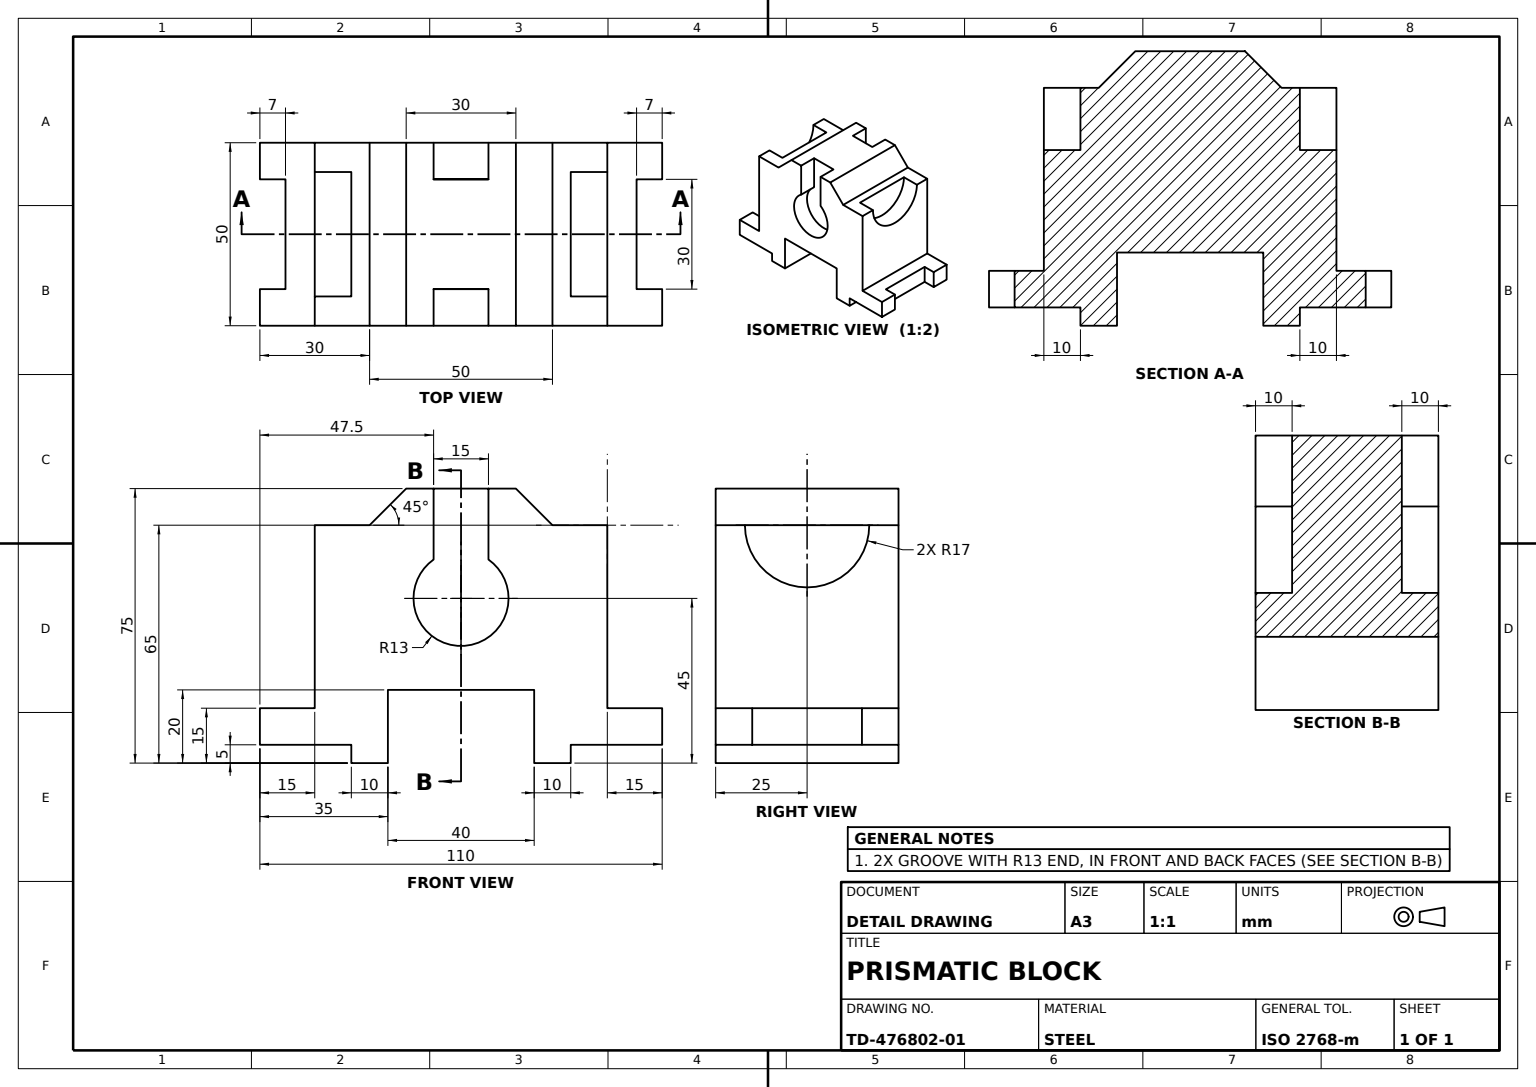
SolidWorks part; units mm, degrees
material "Plain Carbon Steel"
ref_plane "Front Plane" through (0, 0, 0) normal (0, 0, 1) x (1, 0, 0)
ref_plane "Top Plane" through (0, 0, 0) normal (0, 1, 0) x (1, 0, 0)
ref_plane "Right Plane" through (0, 0, 0) normal (1, 0, 0) x (0, 0, -1)
sketch "Body Profile Sketch" plane through (0, 0, 0) normal (0, 0, 1) x (1, 0, 0)
  line L0 (0, 0) -> (0, 5)
  line L1 (0, 5) -> (-25, 5)
  line L2 (0, 0) -> (10, 0)
  line L3 (10, 0) -> (10, 20)
  line L4 (10, 20) -> (50, 20)
  line L5 (50, 20) -> (50, 0)
  line L6 (50, 0) -> (60, 0)
  line L7 (60, 0) -> (60, 5)
  line L8 (60, 5) -> (85, 5)
  line L9 (85, 5) -> (85, 15)
  line L10 (-25, 5) -> (-25, 15)
  line L12 (30, 75) -> (22.5, 75)
  line L13 (30, 75) -> (37.5, 75)
  line L14 (70, 15) -> (70, 65)
  line L15 (70, 65) -> (55, 65)
  line L16 (70, 15) -> (85, 15)
  line L17 (-25, 15) -> (-10, 15)
  line L18 (-10, 15) -> (-10, 65)
  line L19 (-10, 65) -> (5, 65)
  line L20 (22.5, 75) -> (15, 75)
  line L21 (15, 75) -> (5, 65)
  line L22 (37.5, 75) -> (45, 75)
  line L23 (45, 75) -> (55, 65)
  dimension "D1" = 15
  dimension "D2" = 25
  dimension "D3" = 35
  dimension "D4" = 40
  dimension "D5" = 47.5
  dimension "D6" = 5
  dimension "D7" = 20
  dimension "D8" = 65
extrude "Main Body 50mm" add sketch "Body Profile Sketch" along normal blind 50
sketch "Bearing Seat 1 Sketch" plane through (-10, 0, 0) normal (-1, 0, 0) x (0, 0, 1)
  line L0 (50, 65) -> (0, 65) construction
  line L1 (8, 65) -> (42, 65)
  arc A0 (8, 65) -> (42, 65) centre (25, 65) ccw
  dimension "D1" = 17
extrude "Bearing Seat Cut 1" cut sketch "Bearing Seat 1 Sketch" against normal blind 10
sketch "Bearing Seat 2 Sketch" plane through (70, 0, 0) normal (1, 0, 0) x (0, 0, -1)
  line L0 (-50, 65) -> (0, 65) construction
  line L1 (-42, 65) -> (-8, 65)
  arc A0 (-42, 65) -> (-8, 65) centre (-25, 65) ccw
  dimension "D1" = 17
extrude "Bearing Seat Cut 2" cut sketch "Bearing Seat 2 Sketch" against normal blind 10
sketch "Top Groove 1 Sketch" plane through (0, 0, 0) normal (0, 0, -1) x (-1, 0, 0)
  line L0 (25, 15) -> (25, 5) construction
  line L1 (0, 0) -> (-10, 0) construction
  line L2 (-30, 75) -> (-37.5, 75)
  line L3 (-45, 75) -> (-15, 75) construction
  line L4 (-37.5, 75) -> (-37.5, 55.6184)
  line L5 (-30, 75) -> (-22.5, 75)
  line L6 (-22.5, 75) -> (-22.5, 55.6184)
  arc A0 (-37.5, 55.6184) -> (-22.5, 55.6184) centre (-30, 45) ccw
  dimension "D1" = 26
  dimension "D2" = 13
  dimension "D3" = 47.5
  dimension "D4" = 45
extrude "Top Groove Cut 1" cut sketch "Top Groove 1 Sketch" against normal blind 10
sketch "Top Groove 2 Sketch" plane through (0, 0, 50) normal (0, 0, 1) x (1, 0, 0)
  line L0 (85, 5) -> (85, 15) construction
  line L1 (50, 0) -> (60, 0) construction
  line L2 (30, 75) -> (22.5, 75)
  line L3 (45, 75) -> (15, 75) construction
  line L4 (22.5, 75) -> (22.5, 55.6184)
  line L5 (30, 75) -> (37.5, 75)
  line L6 (37.5, 75) -> (37.5, 55.6184)
  arc A0 (22.5, 55.6184) -> (37.5, 55.6184) centre (30, 45) ccw
  dimension "D1" = 26
  dimension "D2" = 13
  dimension "D3" = 47.5
  dimension "D4" = 45
extrude "Top Groove Cut 2" cut sketch "Top Groove 2 Sketch" against normal blind 10
sketch "Base Notch 1 Sketch" plane through (0, 15, 0) normal (0, 1, 0) x (1, 0, 0)
  line L0 (-10, 0) -> (-25, 0) construction
  line L1 (-25, -50) -> (-25, 0) construction
  line L2 (-25, -40) -> (-18, -40)
  line L3 (-18, -40) -> (-18, -10)
  line L4 (-18, -10) -> (-25, -10)
  line L6 (-25, -10) -> (-25, -40)
  dimension "D1" = 7
  dimension "D2" = 10
  dimension "D3" = 40
extrude "Base Notch Cut 1" cut sketch "Base Notch 1 Sketch" against normal blind 10
sketch "Base Notch 2 Sketch" plane through (0, 15, 0) normal (0, 1, 0) x (1, 0, 0)
  line L0 (70, -50) -> (70, 0) construction
  line L1 (85, -50) -> (85, 0) construction
  line L2 (85, -10) -> (78, -10)
  line L3 (78, -10) -> (78, -40)
  line L4 (78, -40) -> (85, -40)
  line L5 (85, -40) -> (85, -10)
  line L6 (85, 0) -> (70, 0) construction
  dimension "D1" = 8
  dimension "D2" = 10
  dimension "D3" = 40
extrude "Base Notch Cut 2" cut sketch "Base Notch 2 Sketch" against normal blind 10
